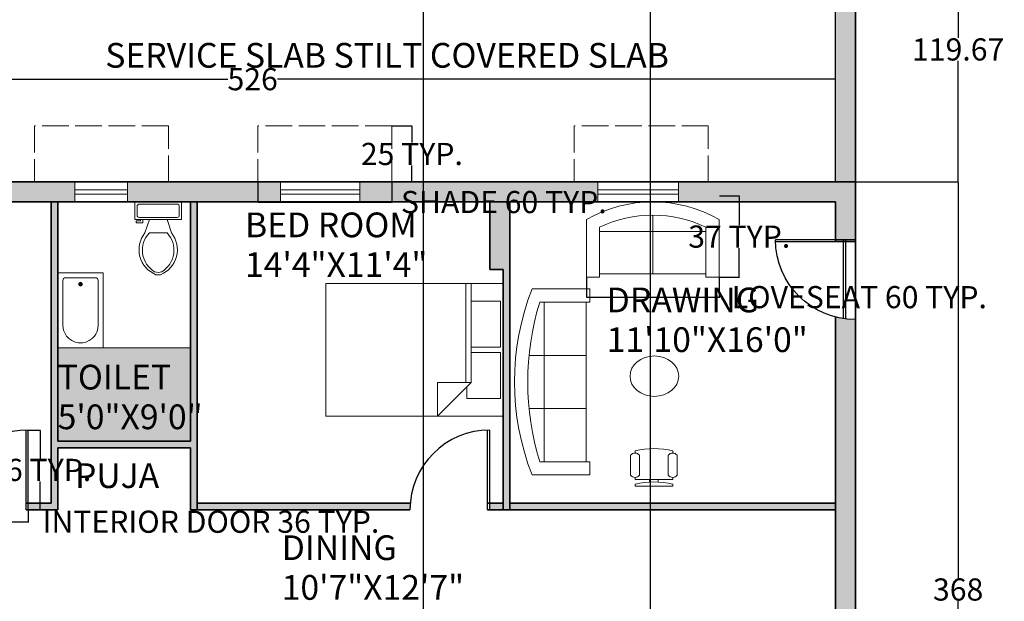
# Model space of a CAD drawing. Units: inches. Extents: x 215 to 969, y -612 to 418.
# Tile 3 of 8: x 502 to 947, y -356 to -93. Entities that reach past the tile are written whole.
import ezdxf

# ---------------------------------------------------------------- set-up
doc = ezdxf.new("R2010")
doc.units = ezdxf.units.IN
doc.header["$MEASUREMENT"] = 0
doc.linetypes.add('ACAD_ISO02W100', pattern=[15, 12, -3])
for name, color, linetype, lineweight in [('A-ANNO-DIMS', 2, 'Continuous', 18), ('A-ANNO-TEXT', 7, 'Continuous', 18), ('A-AREA-IDEN', 7, 'Continuous', 18), ('A-DOOR', 3, 'Continuous', 25), ('A-FLOR-FIXT', 9, 'Continuous', 18), ('A-FLOR-OVHD', 8, 'ACAD_ISO02W100', 13), ('A-FLOR-SLAB', 7, 'Continuous', 25), ('A-FURN', 8, 'Continuous', 18), ('A-GLAZ', 4, 'Continuous', 18), ('A-WALL', 7, 'Continuous', 35)]:
    doc.layers.add(name, color=color, linetype=linetype, lineweight=lineweight)
doc.layers.add('A-WALL-PATT', color=252, linetype='Continuous', lineweight=13, true_color=0x939598)
doc.styles.get("Standard").update_dxf_attribs({"font": 'arial.ttf'})
doc.dimstyles.get("Standard").update_dxf_attribs({"dimtxt": 10, "dimasz": 0.18, "dimexe": 0.18, "dimexo": 0.0625, "dimgap": 0.09, "dimtad": 0, "dimtih": 1, "dimtoh": 1, "dimdec": 0, "dimzin": 0, "dimdsep": 46, "dimlunit": 3, "dimtxsty": 'Standard', "dimcen": 0.09, "dimadec": 0, "dimazin": 0, "dimtfac": 1, "dimtdec": 0, "dimtofl": 0, "dimtmove": 0, "dimatfit": 3, "dimfxl": 1, "dimtolj": 1, "dimtzin": 0, "dimarcsym": 0})

# ---------------------------------------------------------------- blocks, each defined once
blk = doc.blocks.new('Toilet - top')
for p, q in [((9.5, -6), (9.5, -2)), ((-10, -8.5), (-8, -8.5)), ((-10, -9.5), (-10, -8.5)), ((-8, -8.5), (-8, -8)), ((-7, -8), (-7, -9.5)), ((-4, -8), (-6, -14)), ((4, -8), (6, -14)), ((-7, -9.5), (-10, -9.5)), ((4, -14), (-4, -14))]:
    blk.add_line(p, q)
blk.add_lwpolyline([(10.5, -8), (10.5, 0), (-10.5, 0), (-10.5, -8)], close=True)
for points in [[(-9.5, -2), (-9.5, -6)], [(8.5, -1), (-8.5, -1)], [(-8.5, -7), (8.5, -7)]]:
    blk.add_lwpolyline(points)
for centre, radius, start, end in [((-8.62, -1.88), 0.884, 81.8699, 188.1301), ((8.62, -1.88), 0.884, 351.8699, 98.1301), ((-8.62, -6.12), 0.884, 171.8699, 278.1301), ((8.62, -6.12), 0.884, 261.8699, 8.1301), ((3.52, -21.58), 12.17, 141.4691, 247.9714), ((4.2, -21.82), 11.33, 136.3677, 238.9468), ((-3.52, -21.58), 12.17, 292.0284, 38.5307), ((-4.2, -21.82), 11.33, 301.053, 43.6321), ((0, -27.88), 4, 245.7318, 294.2682), ((0, -29), 4, 254.8605, 285.1395)]:
    blk.add_arc(centre, radius, start, end)
blk = doc.blocks.new('Bath Tub - 26 x 60 in.')
for p, q in [((8, -18), (10, -18)), ((9, -17), (9, -19))]:
    blk.add_line(p, q)
blk.add_lwpolyline([(0, -36), (0, 0), (60, 0), (60, -36)], close=True)
for points in [[(4, -30), (4, -6)], [(6, -4), (42, -4)], [(42, -32), (6, -32)]]:
    blk.add_lwpolyline(points)
for radius in [1.5, 1]:
    blk.add_circle((9, -18), radius)
for centre, radius, start, end in [((5.75, -5.75), 1.77, 81.8699, 188.1301), ((42, -18), 14, 270, 90), ((5.75, -30.25), 1.77, 171.8699, 278.1301)]:
    blk.add_arc(centre, radius, start, end)
blk = doc.blocks.new('Bed - Queen')
for p, q in [((0, -80.00003), (0, 0)), ((0, 0), (59.99999, 0)), ((59.99999, 0), (59.99999, -80.00003)), ((7.99999, -1.2), (28.79998, -1.2)), ((7.99999, -14.4), (7.99999, -1.2)), ((28.79998, -1.2), (28.79998, -14.4)), ((31.19999, -1.2), (51.99999, -1.2)), ((31.19999, -14.4), (31.19999, -1.2)), ((51.99999, -1.2), (51.99999, -16.4)), ((0, -14.4), (44.8, -14.4)), ((44.8, -16.8), (0, -16.8)), ((59.99999, -29.6), (44.8, -14.4)), ((44.8, -14.4), (44.8, -29.6)), ((51.99999, -16.4), (46.79936, -16.4)), ((44.8, -29.6), (59.99999, -29.6)), ((59.99999, -80.00003), (0, -80.00003))]:
    blk.add_line(p, q)
blk = doc.blocks.new('Sofa - Roundback 7 ft.')
for p, q in [((-12.00002, -32.4421), (-12.00003, -6.5971)), ((11.99997, -32.4421), (11.99998, -6.5971)), ((-36.000027, -34), (-36.000027, -11.4696)), ((35.99998, -34), (35.99998, -11.4696)), ((-35.999844, -13.3819), (35.9998, -13.3819)), ((-36.000027, -32.4421), (35.99998, -32.4421))]:
    blk.add_line(p, q)
for points in [[(-36.000027, -34), (-42.000027, -34), (-42.000027, -8)], [(41.99998, -8), (41.99998, -34), (35.99998, -34)]]:
    blk.add_lwpolyline(points)
for centre, radius, start, end in [((0, -114.25), 114.25, 68.43141, 111.5686), ((-0.00001, -127.1968), 121.1968, 72.72033, 107.2797)]:
    blk.add_arc(centre, radius, start, end)
blk = doc.blocks.new('Sofa - Roundback Loveseat 5 ft.')
for p, q in [((0, -32.44198), (0, -5.99998)), ((-24, -33.99998), (-24, -11.46958)), ((24.00004, -33.99998), (24.00004, -11.46958)), ((-23.9998, -13.38178), (23.99986, -13.38178)), ((-24, -32.44198), (24.00004, -32.44198))]:
    blk.add_line(p, q)
for points in [[(-24, -33.99998), (-30, -33.99998), (-30, -7.99998)], [(30.00004, -7.99998), (30.00004, -33.99998), (24.00004, -33.99998)]]:
    blk.add_lwpolyline(points)
for centre, radius, start, end in [((0, -60.24998), 60.24998, 60.13715, 119.8628), ((0, -61.38438), 55.38444, 64.32083, 115.6792)]:
    blk.add_arc(centre, radius, start, end)
blk = doc.blocks.new('Chair - Desk')
for p, q in [((-8.5, 0), (-8.5, -1)), ((-8.5, 0), (8.5, 0)), ((8.5, 0), (8.5, -1)), ((-8.5, -3), (-8.5, -4)), ((-8.5, -3), (8.5, -3)), ((-2, -3), (-2, -1.9355)), ((2, -1.9576), (2, -3)), ((8.5, -3), (8.5, -4)), ((-10.5, -5), (-10.5, -14)), ((-6.5, -14), (-6.5, -5)), ((6.5, -5), (6.5, -14)), ((10.5, -14), (10.5, -5)), ((-8.5, -15), (-8.5, -16)), ((8.5, -15), (8.5, -16))]:
    blk.add_line(p, q)
for centre, radius, start, end in [((-8.5, -6.5), 2.5, 36.8699, 143.1301), ((0, 34.625), 36.625, 256.5803, 283.4197), ((8.5, -6.5), 2.5, 36.8699, 143.1301), ((-8.5, -12.5), 2.5, 216.8699, 323.1301), ((0, 19.625), 36.625, 256.5803, 283.4197), ((8.5, -12.5), 2.5, 216.8699, 323.1301)]:
    blk.add_arc(centre, radius, start, end)
blk = doc.blocks.new('WINDOW-SHADE-60')
for p, q in [((60.48, 25.28), (0, 25.28)), ((0, 25.28), (0, 0)), ((60.48, 0), (60.48, 25.28))]:
    blk.add_line(p, q)
blk = doc.blocks.new('DOOR-SINGLE-36')
for p, q in [((35, 0), (35, 36)), ((36, 0), (36, 36)), ((35, 0), (36, 0))]:
    blk.add_line(p, q)
blk.add_arc((36, 0), 36, 90, 180)
blk = doc.blocks.new('DOOR-ENTRY-36')
for p, q in [((36, 1), (0, 1)), ((36, 0), (0, 0))]:
    blk.add_line(p, q)
blk.add_arc((36, 0), 36, 90, 180)
blk = doc.blocks.new('WIN-FRAME-24A')
for p, q in [((0, 0), (0, 9)), ((23.77, 0), (23.77, 9)), ((23.77, 5.5), (0, 5.5)), ((0, 4.5), (0, 0)), ((23.77, 3.5), (0, 3.5))]:
    blk.add_line(p, q)
blk = doc.blocks.new('WIN-FRAME-36A')
for p, q in [((0, 35.94), (9, 35.94)), ((3.5, 35.94), (3.5, 0)), ((5.5, 35.94), (5.5, 0)), ((9, 0), (0, 0)), ((4.5, 0), (9, 0))]:
    blk.add_line(p, q)
blk = doc.blocks.new('WIN-FRAME-36B')
for p, q in [((9, 36.42), (0, 36.42)), ((3.5, 36.42), (3.5, 0)), ((5.5, 36.42), (5.5, 0)), ((4.5, 0), (0, 0)), ((0, 0), (9, 0))]:
    blk.add_line(p, q)
blk = doc.blocks.new('*D37')
at = {"layer": 'A-ANNO-DIMS', "color": 0, "lineweight": -2, "transparency": 16777216}
for p, q in [((609.64, -166.51), (609.64, -175.7)), ((670.12, -166.51), (670.12, -175.7)), ((609.82, -175.52), (669.94, -175.52)), ((670.12, -175.52), (670.3, -175.52))]:
    blk.add_line(p, q, dxfattribs=at)
at = {"layer": 'A-ANNO-DIMS', "color": 0, "transparency": 16777216}
for points in [[(609.82, -175.49), (609.82, -175.55), (609.64, -175.52)], [(669.94, -175.49), (669.94, -175.55), (670.12, -175.52)]]:
    blk.add_solid(points, dxfattribs=at)
at = {"layer": 'Defpoints', "color": 0, "transparency": 16777216}
for p in [(609.64, -166.45), (670.12, -166.45), (670.12, -175.52)]:
    blk.add_point(p, dxfattribs=at)
at = {"layer": 'A-ANNO-DIMS', "color": 0, "transparency": 16777216, "insert": (720.71, -175.52), "char_height": 10, "attachment_point": 5}
blk.add_mtext('\\A1;SHADE 60 TYP.', dxfattribs=at)
blk = doc.blocks.new('*D38')
at = {"layer": 'A-ANNO-DIMS', "color": 0, "lineweight": -2, "transparency": 16777216}
for p, q in [((670.19, -141.18), (679.38, -141.18)), ((679.2, -141.36), (679.2, -148.62)), ((679.2, -166.27), (679.2, -159.01)), ((670.19, -166.45), (679.38, -166.45))]:
    blk.add_line(p, q, dxfattribs=at)
at = {"layer": 'A-ANNO-DIMS', "color": 0, "transparency": 16777216}
for points in [[(679.17, -141.36), (679.23, -141.36), (679.2, -141.18)], [(679.17, -166.27), (679.23, -166.27), (679.2, -166.45)]]:
    blk.add_solid(points, dxfattribs=at)
at = {"layer": 'Defpoints', "color": 0, "transparency": 16777216}
for p in [(670.12, -141.18), (679.2, -141.18), (670.12, -166.45)]:
    blk.add_point(p, dxfattribs=at)
at = {"layer": 'A-ANNO-DIMS', "color": 0, "transparency": 16777216, "insert": (679.2, -153.81), "char_height": 10, "attachment_point": 5}
blk.add_mtext('\\A1;25 TYP.', dxfattribs=at)
blk = doc.blocks.new('*D39')
at = {"layer": 'A-ANNO-DIMS', "color": 0, "lineweight": -2, "transparency": 16777216}
for p, q in [((470.07, -314.51), (470.07, -320.03)), ((506.07, -314.51), (506.07, -320.03)), ((470.25, -319.85), (505.89, -319.85)), ((506.07, -319.85), (506.25, -319.85))]:
    blk.add_line(p, q, dxfattribs=at)
at = {"layer": 'A-ANNO-DIMS', "color": 0, "transparency": 16777216}
for points in [[(470.25, -319.82), (470.25, -319.88), (470.07, -319.85)], [(505.89, -319.82), (505.89, -319.88), (506.07, -319.85)]]:
    blk.add_solid(points, dxfattribs=at)
at = {"layer": 'Defpoints', "color": 0, "transparency": 16777216}
for p in [(470.07, -314.45), (506.07, -314.45), (506.07, -319.85)]:
    blk.add_point(p, dxfattribs=at)
at = {"layer": 'A-ANNO-DIMS', "color": 0, "transparency": 16777216, "insert": (588.53, -319.85), "char_height": 10, "attachment_point": 5}
blk.add_mtext('\\A1;INTERIOR DOOR 36 TYP.', dxfattribs=at)
blk = doc.blocks.new('*D40')
at = {"layer": 'A-ANNO-DIMS', "color": 0, "lineweight": -2, "transparency": 16777216}
for p, q in [((506.13, -278.45), (511.65, -278.45)), ((511.47, -278.63), (511.47, -291.25)), ((511.47, -314.27), (511.47, -301.65)), ((506.13, -314.45), (511.65, -314.45))]:
    blk.add_line(p, q, dxfattribs=at)
at = {"layer": 'A-ANNO-DIMS', "color": 0, "transparency": 16777216}
for points in [[(511.44, -278.63), (511.5, -278.63), (511.47, -278.45)], [(511.44, -314.27), (511.5, -314.27), (511.47, -314.45)]]:
    blk.add_solid(points, dxfattribs=at)
at = {"layer": 'Defpoints', "color": 0, "transparency": 16777216}
for p in [(506.07, -278.45), (511.47, -278.45), (506.07, -314.45)]:
    blk.add_point(p, dxfattribs=at)
at = {"layer": 'A-ANNO-DIMS', "color": 0, "transparency": 16777216, "insert": (511.47, -296.45), "char_height": 10, "attachment_point": 5}
blk.add_mtext('\\A1;36 TYP.', dxfattribs=at)
blk = doc.blocks.new('*D43')
at = {"layer": 'A-ANNO-DIMS', "color": 0, "lineweight": -2, "transparency": 16777216}
for p, q in [((757.95, -209.51), (757.95, -218.63)), ((817.95, -209.51), (817.95, -218.63)), ((758.13, -218.45), (817.77, -218.45)), ((817.95, -218.45), (818.13, -218.45))]:
    blk.add_line(p, q, dxfattribs=at)
at = {"layer": 'A-ANNO-DIMS', "color": 0, "transparency": 16777216}
for points in [[(758.13, -218.42), (758.13, -218.48), (757.95, -218.45)], [(817.77, -218.42), (817.77, -218.48), (817.95, -218.45)]]:
    blk.add_solid(points, dxfattribs=at)
at = {"layer": 'Defpoints', "color": 0, "transparency": 16777216}
for p in [(757.95, -209.45), (817.95, -209.45), (817.95, -218.45)]:
    blk.add_point(p, dxfattribs=at)
at = {"layer": 'A-ANNO-DIMS', "color": 0, "transparency": 16777216, "insert": (881.15, -218.45), "char_height": 10, "attachment_point": 5}
blk.add_mtext('\\A1;LOVESEAT 60 TYP.', dxfattribs=at)
blk = doc.blocks.new('*D44')
at = {"layer": 'A-ANNO-DIMS', "color": 0, "lineweight": -2, "transparency": 16777216}
for p, q in [((818.01, -172.79), (827.13, -172.79)), ((826.95, -172.97), (826.95, -185.92)), ((826.95, -209.27), (826.95, -196.32)), ((818.01, -209.45), (827.13, -209.45))]:
    blk.add_line(p, q, dxfattribs=at)
at = {"layer": 'A-ANNO-DIMS', "color": 0, "transparency": 16777216}
for points in [[(826.92, -172.97), (826.98, -172.97), (826.95, -172.79)], [(826.92, -209.27), (826.98, -209.27), (826.95, -209.45)]]:
    blk.add_solid(points, dxfattribs=at)
at = {"layer": 'Defpoints', "color": 0, "transparency": 16777216}
for p in [(817.95, -172.79), (826.95, -172.79), (817.95, -209.45)]:
    blk.add_point(p, dxfattribs=at)
at = {"layer": 'A-ANNO-DIMS', "color": 0, "transparency": 16777216, "insert": (826.95, -191.12), "char_height": 10, "attachment_point": 5}
blk.add_mtext('\\A1;37 TYP.', dxfattribs=at)
blk = doc.blocks.new('*D69')
at = {"layer": 'A-ANNO-DIMS', "color": 0, "lineweight": -2, "transparency": 16777216}
for p, q in [((344.35, -166.39), (344.35, -119.87)), ((870.35, -166.39), (870.35, -119.87)), ((344.53, -120.05), (596.22, -120.05)), ((870.17, -120.05), (618.49, -120.05))]:
    blk.add_line(p, q, dxfattribs=at)
at = {"layer": 'A-ANNO-DIMS', "color": 0, "transparency": 16777216}
for points in [[(344.53, -120.02), (344.53, -120.08), (344.35, -120.05)], [(870.17, -120.02), (870.17, -120.08), (870.35, -120.05)]]:
    blk.add_solid(points, dxfattribs=at)
at = {"layer": 'Defpoints', "color": 0, "transparency": 16777216}
for p in [(870.35, -120.05), (344.35, -166.45), (870.35, -166.45)]:
    blk.add_point(p, dxfattribs=at)
at = {"layer": 'A-ANNO-DIMS', "color": 0, "transparency": 16777216, "insert": (607.35, -120.05), "char_height": 10, "attachment_point": 5}
blk.add_mtext('\\A1;526', dxfattribs=at)
blk = doc.blocks.new('*D71')
at = {"layer": 'A-ANNO-DIMS', "color": 0, "lineweight": -2, "transparency": 16777216}
for p, q in [((879.42, -46.79), (925.93, -46.79)), ((925.75, -46.97), (925.75, -101.42)), ((925.75, -166.27), (925.75, -111.82)), ((879.42, -166.45), (925.93, -166.45))]:
    blk.add_line(p, q, dxfattribs=at)
at = {"layer": 'A-ANNO-DIMS', "color": 0, "transparency": 16777216}
for points in [[(925.72, -46.97), (925.78, -46.97), (925.75, -46.79)], [(925.72, -166.27), (925.78, -166.27), (925.75, -166.45)]]:
    blk.add_solid(points, dxfattribs=at)
at = {"layer": 'Defpoints', "color": 0, "transparency": 16777216}
for p in [(879.35, -46.79), (879.35, -166.45), (925.75, -166.45)]:
    blk.add_point(p, dxfattribs=at)
at = {"layer": 'A-ANNO-DIMS', "color": 0, "transparency": 16777216, "insert": (925.75, -106.62), "char_height": 10, "attachment_point": 5}
blk.add_mtext('\\A1;119.67', dxfattribs=at)
blk = doc.blocks.new('*D72')
at = {"layer": 'A-ANNO-DIMS', "color": 0, "lineweight": -2, "transparency": 16777216}
for p, q in [((879.42, -166.45), (925.93, -166.45)), ((925.75, -166.63), (925.75, -345.25)), ((925.75, -534.27), (925.75, -355.65)), ((879.42, -534.45), (925.93, -534.45))]:
    blk.add_line(p, q, dxfattribs=at)
at = {"layer": 'A-ANNO-DIMS', "color": 0, "transparency": 16777216}
for points in [[(925.72, -166.63), (925.78, -166.63), (925.75, -166.45)], [(925.72, -534.27), (925.78, -534.27), (925.75, -534.45)]]:
    blk.add_solid(points, dxfattribs=at)
at = {"layer": 'Defpoints', "color": 0, "transparency": 16777216}
for p in [(879.35, -166.45), (879.35, -534.45), (925.75, -534.45)]:
    blk.add_point(p, dxfattribs=at)
at = {"layer": 'A-ANNO-DIMS', "color": 0, "transparency": 16777216, "insert": (925.75, -350.45), "char_height": 10, "attachment_point": 5}
blk.add_mtext('\\A1;368', dxfattribs=at)
blk = doc.blocks.new('*D75')
at = {"layer": 'A-ANNO-DIMS', "color": 0, "lineweight": -2, "transparency": 16777216}
for p, q in [((290.35, 103.15), (290.35, -605.89)), ((879.35, -534.51), (879.35, -605.89)), ((290.53, -605.71), (573.71, -605.71)), ((879.17, -605.71), (596, -605.71))]:
    blk.add_line(p, q, dxfattribs=at)
at = {"layer": 'A-ANNO-DIMS', "color": 0, "transparency": 16777216}
for points in [[(290.53, -605.68), (290.53, -605.74), (290.35, -605.71)], [(879.17, -605.68), (879.17, -605.74), (879.35, -605.71)]]:
    blk.add_solid(points, dxfattribs=at)
at = {"layer": 'Defpoints', "color": 0, "transparency": 16777216}
for p in [(290.35, 103.21), (879.35, -534.45), (879.35, -605.71)]:
    blk.add_point(p, dxfattribs=at)
at = {"layer": 'A-ANNO-DIMS', "color": 0, "transparency": 16777216, "insert": (584.85, -605.71), "char_height": 10, "attachment_point": 5}
blk.add_mtext('\\A1;589', dxfattribs=at)
blk = doc.blocks.new('*D76')
at = {"layer": 'A-ANNO-DIMS', "color": 0, "lineweight": -2, "transparency": 16777216}
for p, q in [((569.29, 365.5), (243.77, 365.5)), ((243.95, 365.32), (243.95, -91.71)), ((243.95, -559.13), (243.95, -102.1)), ((454.66, -559.31), (243.77, -559.31))]:
    blk.add_line(p, q, dxfattribs=at)
at = {"layer": 'A-ANNO-DIMS', "color": 0, "transparency": 16777216}
for points in [[(243.92, 365.32), (243.98, 365.32), (243.95, 365.5)], [(243.92, -559.13), (243.98, -559.13), (243.95, -559.31)]]:
    blk.add_solid(points, dxfattribs=at)
at = {"layer": 'Defpoints', "color": 0, "transparency": 16777216}
for p in [(569.35, 365.5), (243.95, -559.31), (454.72, -559.31)]:
    blk.add_point(p, dxfattribs=at)
at = {"layer": 'A-ANNO-DIMS', "color": 0, "transparency": 16777216, "insert": (243.95, -96.91), "char_height": 10, "attachment_point": 5}
blk.add_mtext('\\A1;924.8', dxfattribs=at)
blk = doc.blocks.new('*D79')
at = {"layer": 'A-ANNO-DIMS', "color": 0, "lineweight": -2, "transparency": 16777216}
for p, q in [((684.35, -82.85), (684.35, -605.89)), ((786.74, -82.85), (786.74, -605.89)), ((684.53, -605.71), (715.16, -605.71)), ((786.56, -605.71), (755.93, -605.71))]:
    blk.add_line(p, q, dxfattribs=at)
at = {"layer": 'A-ANNO-DIMS', "color": 0, "transparency": 16777216}
for points in [[(684.53, -605.68), (684.53, -605.74), (684.35, -605.71)], [(786.56, -605.68), (786.56, -605.74), (786.74, -605.71)]]:
    blk.add_solid(points, dxfattribs=at)
at = {"layer": 'Defpoints', "color": 0, "transparency": 16777216}
for p in [(684.35, -82.79), (786.74, -82.79), (786.74, -605.71)]:
    blk.add_point(p, dxfattribs=at)
at = {"layer": 'A-ANNO-DIMS', "color": 0, "transparency": 16777216, "insert": (735.55, -605.71), "char_height": 10, "attachment_point": 5}
blk.add_mtext('\\A1;102.38', dxfattribs=at)
blk = doc.blocks.new('*D81')
at = {"layer": 'A-ANNO-DIMS', "color": 0, "lineweight": -2, "transparency": 16777216}
for p, q in [((786.74, -46.85), (786.74, -605.89)), ((879.35, -46.85), (879.35, -605.89)), ((786.92, -605.71), (816.13, -605.71)), ((879.17, -605.71), (849.96, -605.71))]:
    blk.add_line(p, q, dxfattribs=at)
at = {"layer": 'A-ANNO-DIMS', "color": 0, "transparency": 16777216}
for points in [[(786.92, -605.68), (786.92, -605.74), (786.74, -605.71)], [(879.17, -605.68), (879.17, -605.74), (879.35, -605.71)]]:
    blk.add_solid(points, dxfattribs=at)
at = {"layer": 'Defpoints', "color": 0, "transparency": 16777216}
for p in [(786.74, -46.79), (879.35, -46.79), (879.35, -605.71)]:
    blk.add_point(p, dxfattribs=at)
at = {"layer": 'A-ANNO-DIMS', "color": 0, "transparency": 16777216, "insert": (833.05, -605.71), "char_height": 10, "attachment_point": 5}
blk.add_mtext('\\A1;92.62', dxfattribs=at)

msp = doc.modelspace()

# ---------------------------------------------------------------- hatches: boundary and pattern name
at = {"layer": 'A-WALL-PATT'}
h = msp.add_hatch(color=256, dxfattribs=at)
h.dxf.hatch_style = 1
h.paths.add_polyline_path([(764.0736, 322.2135), (569.3535, 322.2135), (565.0643, 322.2135), (565.0643, 313.2135), (569.3535, 313.2135), (569.3535, 205.2135), (509.3535, 205.2135), (509.3535, 247.2592), (506.3535, 247.2592), (506.3535, 172.2135), (491.3535, 172.2135), (491.3535, 169.2135), (509.3535, 169.2135), (509.3535, 202.2135), (569.3535, 202.2135), (569.3535, 169.2135), (578.3535, 169.2135), (578.3535, 205.2135), (578.3535, 237.2135), (615.7789, 237.2135), (615.7789, 246.2135), (578.3535, 246.2135), (578.3535, 313.2135), (710.3535, 313.2135), (710.3535, 246.2135), (710.3535, 211.3874), (719.3535, 211.3874), (719.3535, 295.2135), (719.3535, 313.2135), (764.0736, 313.2135)])
h.paths.add_polyline_path([(879.3535, 322.2135), (811.6486, 322.2135), (811.6486, 313.2135), (870.3535, 313.2135), (870.3535, 215.3905, -0.06325422), (879.3535, 216.5337), (879.3535, 313.2135)])
h.paths.add_polyline_path([(879.3535, 157.2135), (879.3535, 180.5337), (870.3535, 180.5337), (870.3535, 157.2135), (719.3535, 157.2135), (710.3535, 157.2135), (710.3535, 148.2135), (719.3535, 148.2135), (870.3535, 148.2135), (870.3535, 16.2135), (838.4933, 16.2135), (838.4933, 13.2135), (870.3535, 13.2135), (870.3535, -37.7865), (844.0345, -37.7865), (844.0345, -46.7865), (870.3535, -46.7865), (879.3535, -46.7865), (879.3535, -37.7865), (879.3535, 137.613)])
h.paths.add_polyline_path([(710.3535, 246.2135), (663.4146, 246.2135), (663.4146, 237.2135), (710.3535, 237.2135)], flags=17)
h.paths.add_polyline_path([(541.2942, 322.2135), (509.3535, 322.2135), (468.3222, 322.2135), (468.3222, 313.2135), (500.3535, 313.2135), (509.3535, 313.2135), (541.2942, 313.2135)])
h.paths.add_polyline_path([(509.3535, 313.2135), (503.3535, 313.2135), (503.3535, 277.5241, -0.04952579), (509.3535, 277.4203)], flags=17)
h.paths.add_polyline_path([(420.2828, 322.2135), (335.3535, 322.2135), (335.3535, 235.2487), (344.3535, 235.2487), (344.3535, 284.1885), (344.3535, 313.2135), (420.2828, 313.2135)])
h.paths.add_polyline_path([(335.3535, 181.2135), (290.3535, 181.2135), (290.3535, 103.2135), (335.3535, 103.2135), (335.3535, 112.2135), (299.3535, 112.2135), (299.3535, 129.1615), (299.3535, 172.2135), (335.3535, 172.2135)])
h.paths.add_polyline_path([(344.3535, 199.3097), (335.3535, 199.3097), (335.3535, 172.2135), (335.3535, 157.3369), (344.3535, 157.3369), (344.3535, 169.2135), (452.3535, 169.2135), (452.5037, 169.2135), (452.5037, 150.1199), (452.3535, 109.2135), (455.3535, 109.2135), (455.3535, 169.2135, -0.02086055), (455.4787, 172.2135), (344.3535, 172.2135)])
h.paths.add_polyline_path([(344.3535, 133.3441), (335.3535, 133.3441), (335.3535, 77.89), (344.3535, 77.89), (344.3535, 103.2135), (401.3556, 103.2135), (401.3556, 109.2135), (344.3535, 109.2135)])
h.paths.add_polyline_path([(462.6362, 109.2135), (443.0437, 109.2135), (425.2018, 109.2135), (425.2018, 106.2135), (452.3535, 106.2135), (462.7615, 106.2135, -0.02086055)])
h.paths.add_polyline_path([(540.3535, 106.2135), (684.3535, 106.2135), (684.3535, 35.7135), (687.3535, 35.7135), (687.3535, 56.1856), (693.3535, 56.1856), (693.3535, 109.2135), (540.3535, 109.2135), (531.3535, 109.2135), (498.6362, 109.2135), (498.6362, 106.2135), (531.3535, 106.2135), (531.3535, -37.7865), (507.9524, -37.7865), (507.9524, -46.7865), (610.6038, -46.7865), (610.6038, -37.7865), (540.3535, -37.7865)])
h.paths.add_polyline_path([(578.3535, 358.6622), (555.879, 358.6622), (555.879, 349.6622), (569.3535, 349.6622), (569.3535, 322.2135), (578.3535, 322.2135)])
h.paths.add_polyline_path([(525.962, 358.6622), (503.3535, 358.6622), (503.3535, 322.2135), (509.3535, 322.2135), (509.3535, 349.6622), (525.962, 349.6622)])
h.paths.add_polyline_path([(344.3535, 30.022), (335.3535, 30.022), (335.3535, -37.7865), (335.3535, -46.7865), (484.3302, -46.7865), (484.3302, -37.7865), (344.3535, -37.7865)])
h.paths.add_polyline_path([(719.1188, -37.7865), (698.4193, -37.7865), (693.3535, -37.7865), (693.3535, 7.424, -0.07717369), (684.3535, 6.0404), (684.3535, -37.7865), (658.8269, -37.7865), (658.8269, -46.7865), (684.3535, -46.7865), (684.3535, -82.7865), (693.3535, -82.7865), (704.1236, -82.7865), (704.1236, -78.0462), (693.3535, -78.0462), (693.3535, -46.7865), (719.1188, -46.7865)])
h.paths.add_polyline_path([(684.3535, -14.2202), (669.6716, -14.2202), (669.6716, -16.6044, -0.23606798), (667.6716, -17.6044), (667.6716, -18.6044, -0.11764706), (650.6716, -18.6044), (650.6716, -17.6044, -0.23606798), (648.6716, -16.6044), (648.6716, -14.2202), (603.0565, -14.2202), (603.0565, -37.7865), (684.3535, -37.7865)], flags=17)
h.paths.add_polyline_path([(665.6716, -14.2202), (652.6716, -14.2202), (652.6716, -16.6044, -0.23606798), (650.6716, -17.6044), (650.6716, -18.6044, 0.11764706), (667.6716, -18.6044), (667.6716, -17.6044, -0.23606798), (665.6716, -16.6044)], flags=16)
h.paths.add_polyline_path([(786.7385, -37.7865), (755.3535, -37.7865), (755.3535, 13.2135), (769.0808, 13.2135), (769.0808, 16.2135), (755.3535, 16.2135), (755.3535, 73.2135), (753.3535, 73.2135), (693.3535, 73.2135), (693.3535, 70.2135), (753.3535, 70.2135), (753.3535, -37.7865), (743.3062, -37.7865), (743.3062, -46.7865), (781.7385, -46.7865), (781.7385, -82.7865), (786.7385, -82.7865), (786.7385, -82.3744), (786.7385, -46.7865)])
h.paths.add_polyline_path([(844.0345, -37.7865), (786.7385, -37.7865), (786.7385, -46.7865), (844.0345, -46.7865)], flags=17)
h.paths.add_polyline_path([(781.7385, -78.0462), (704.1236, -78.0462), (704.1236, -82.7865), (781.7385, -82.7865)], flags=17)
h.paths.add_polyline_path([(344.3535, -46.7865), (335.3535, -46.7865), (335.3535, -166.4525), (344.3535, -166.4525)])
h.paths.add_polyline_path([(382.6632, 103.2135), (344.3535, 103.2135), (344.3535, 77.89), (344.3535, 32.7135), (363.5083, 32.7135), (382.6632, 32.7135)])
h.paths.add_polyline_path([(879.3535, -46.7865), (870.3535, -46.7865), (870.3535, -166.4525), (879.3535, -166.4525)])
h.paths.add_polyline_path([(879.3535, -166.4525), (799.4745, -166.4525), (799.4745, -175.4525), (855.3535, -175.4525), (870.3535, -175.4525), (870.3535, -192.5449), (879.3535, -192.5449), (879.3535, -175.4525)])
h.paths.add_polyline_path([(763.1775, -166.4525), (655.7214, -166.4525), (655.7214, -175.4525), (763.1775, -175.4525)])
h.paths.add_polyline_path([(619.8538, -166.4525), (550.8369, -166.4525), (550.8369, -175.4525), (619.8538, -175.4525)])
h.paths.add_polyline_path([(527.1282, -166.4525), (427.0819, -166.4525), (427.0819, -175.4525), (527.1282, -175.4525)])
h.paths.add_polyline_path([(391.4021, -166.4525), (335.3535, -166.4525), (335.3535, -175.4525), (335.3535, -236.0109), (344.3535, -236.0109), (344.3535, -187.5037), (344.3535, -175.4525), (391.4021, -175.4525)])
h.paths.add_polyline_path([(344.3535, -271.9249), (335.3535, -271.9249), (335.3535, -331.0209), (344.3535, -331.0209), (344.3535, -314.4525), (412.4218, -314.4525, -0.02503209), (412.3073, -311.4525), (344.3535, -311.4525)])
h.paths.add_polyline_path([(470.1954, -311.4525), (442.3073, -311.4525), (442.3073, -314.4525), (470.0702, -314.4525, -0.02086055)])
h.paths.add_polyline_path([(455.3535, -314.4525), (452.3535, -314.4525), (452.3535, -374.4525), (455.3535, -374.4525)])
h.paths.add_polyline_path([(579.3535, -241.4072), (519.3535, -241.4072), (519.3535, -283.4525), (579.3535, -283.4525)])
h.paths.add_polyline_path([(516.5043, -281.1089), (584.3098, -281.1089), (584.3098, -264.0138), (516.5043, -264.0138)], flags=9)
h.paths.add_polyline_path([(516.4662, -263.2183), (581.1504, -263.2183), (581.1504, -245.8948), (516.4662, -245.8948)], flags=9)
h = msp.add_hatch(color=256, dxfattribs=at)
h.dxf.hatch_style = 1
h.paths.add_polyline_path([(723.3535, -175.4525), (714.3535, -175.4525), (714.3535, -205.9065), (720.3535, -205.9065), (720.3535, -314.4525), (723.3535, -314.4525)])
h.paths.add_polyline_path([(720.3535, -311.4525), (714.3535, -311.4525), (714.3535, -314.4525), (720.3535, -314.4525)], flags=17)
h.paths.add_polyline_path([(879.3535, -228.5449, -0.06325422), (870.3535, -227.4017), (870.3535, -314.4525), (870.3535, -410.4525), (870.3535, -464.8456), (870.3535, -525.4525), (730.3535, -525.4525), (730.3535, -473.8456), (753.1403, -473.8456), (753.1403, -464.8456), (686.9324, -464.8456), (686.9324, -473.8456), (721.3535, -473.8456), (721.3535, -525.4525), (594.3535, -525.4525), (594.3535, -473.8456), (622.1543, -473.8456), (622.1543, -464.8456), (594.3535, -464.8456), (594.3535, -414.4525), (525.3535, -414.4525), (525.3535, -417.4525), (585.3535, -417.4525), (585.3535, -525.4525), (571.9682, -525.4525), (571.9682, -534.4525), (879.3535, -534.4525), (879.3535, -410.4525), (879.3535, -314.4525)])
h.paths.add_polyline_path([(730.3535, -368.8456), (870.3535, -368.8456), (870.3535, -365.8456), (721.3535, -365.8456), (721.3535, -368.8456), (721.3535, -409.1143), (730.3535, -409.1143)], flags=17)
h.paths.add_polyline_path([(870.3535, -410.4525), (870.3535, -368.8456), (763.5487, -368.8456), (763.5487, -393.1792), (831.3894, -393.1792), (831.3894, -438.7284), (789.7386, -438.7284), (789.7386, -464.8456), (870.3535, -464.8456)], flags=17)
h.paths.add_polyline_path([(839.0857, -434.8848), (839.0857, -399.5193), (865.1757, -399.5193), (865.1757, -434.8848)], flags=16)
h.paths.add_polyline_path([(839.8092, -427.6923, -0.48074962), (841.3551, -426.456, -0.48074962), (842.901, -427.6923, -0.48074962), (841.3551, -428.9285, -0.48074962)], flags=0)
h.paths.add_polyline_path([(848.5001, -427.1588, -0.44021274), (854.7228, -421.4606, -0.49540019), (861.9637, -426.9752, -0.44021274), (855.741, -432.6734, -0.49540019)], flags=0)
h.paths.add_polyline_path([(848.5001, -410.0762, -0.44021274), (854.7228, -404.378, -0.49540019), (861.9637, -409.8925, -0.44021274), (855.741, -415.5907, -0.49540019)], flags=0)
h.paths.add_polyline_path([(839.8092, -410.149, -0.48074962), (841.3551, -408.9127, -0.48074962), (842.901, -410.149, -0.48074962), (841.3551, -411.3852, -0.48074962)], flags=0)
h.paths.add_polyline_path([(870.3535, -464.8456), (789.7386, -464.8456), (789.1403, -464.8456, -0.06325422), (787.9971, -473.8456), (870.3535, -473.8456)], flags=17)
h.paths.add_polyline_path([(727.9401, -444.9303), (724.3796, -444.9303), (724.3796, -464.8456), (727.9401, -464.8456)], flags=17)
h.paths.add_polyline_path([(548.597, -525.4525), (531.2503, -525.4525), (525.3535, -525.4525), (525.3535, -490.3641, -0.07632083), (516.3535, -491.7459), (516.3535, -525.4525), (488.9462, -525.4525), (488.9462, -534.4525), (548.597, -534.4525)])
h.paths.add_polyline_path([(525.3535, -374.4525), (506.0702, -374.4525), (506.0702, -377.4525), (516.3535, -377.4525), (516.3535, -461.7459), (519.3535, -461.7459), (519.3535, -417.4525), (525.3535, -417.4525), (525.3535, -414.4525)])
h.paths.add_polyline_path([(470.1724, -377.4525), (449.6899, -377.4525), (344.3535, -377.4525), (344.3535, -400.7118), (335.3535, -400.7118), (335.3535, -355.0472), (344.3535, -355.0472), (344.3535, -374.4525), (373.6368, -374.4525), (373.6368, -366.4525), (380.1368, -366.4525), (378.1369, -360.4526, -0.50132349), (383.0921, -341.5914, -0.13289091), (385.1815, -341.5914, -0.50131678), (390.1369, -360.4524), (388.1368, -366.4525), (391.1368, -366.4525), (391.1368, -364.9525), (394.1368, -364.9525), (394.1368, -365.9525), (392.1368, -365.9525), (392.1368, -366.4525), (394.6368, -366.4525), (394.6368, -374.4525), (418.4066, -374.4525), (418.4066, -354.0926), (452.3535, -354.0926), (452.3535, -374.4525), (470.0713, -374.4525, 0.02085422)])
h.paths.add_polyline_path([(442.1598, -372.1903), (421.7999, -372.1903, -0.50000012), (420.6688, -371.0592), (420.6688, -357.4859, -0.50000012), (421.7999, -356.3548), (442.1598, -356.3548, -1)], flags=16)
h.paths.add_polyline_path([(422.6483, -364.2725, -1), (424.3449, -364.2725, -1)], flags=0)
h.paths.add_polyline_path([(422.931, -364.2725, -1), (424.0621, -364.2725, -1)], flags=0)
h.paths.add_polyline_path([(392.6368, -373.4525), (375.6368, -373.4525, -0.50000012), (374.6368, -372.4525), (374.6368, -368.4525, -0.50000012), (375.6368, -367.4525), (392.6368, -367.4525, -0.50000012), (393.6368, -368.4525), (393.6368, -372.4525, -0.50000012)], flags=16)
h.paths.add_polyline_path([(388.1368, -360.4525), (380.1368, -360.4525, -0.4800795), (382.4928, -342.9295, -0.21500378), (385.7809, -342.9295, -0.48007965)], flags=16)
h.paths.add_polyline_path([(344.3535, -437.1356), (335.3535, -437.1356), (335.3535, -525.4525), (335.3535, -534.4525), (465.575, -534.4525), (465.575, -525.4525), (344.3535, -525.4525)])
h.paths.add_polyline_path([(342.2824, -347.0067), (391.5718, -347.0067), (391.5718, -334.5799), (342.2824, -334.5799)], flags=9)
h = msp.add_hatch(color=256, dxfattribs=at)
h.dxf.hatch_style = 1
h.paths.add_polyline_path([(678.4787, -311.4525), (582.3535, -311.4525), (582.3535, -314.4525), (678.3535, -314.4525, -0.02086055)])
h.paths.add_polyline_path([(582.3535, -283.4525), (582.3535, -175.4525), (579.3535, -175.4525), (579.3535, -283.4525), (519.3535, -283.4525), (519.3535, -175.4525), (516.3535, -175.4525), (516.3535, -311.4525), (506.0702, -311.4525), (506.0702, -314.4525), (519.3535, -314.4525), (519.3535, -286.4525), (579.3535, -286.4525), (579.3535, -314.4525), (582.3535, -314.4525), (582.3535, -311.4525)])
h.paths.add_polyline_path([(870.3535, -311.4525), (723.3535, -311.4525), (723.3535, -314.4525), (870.3535, -314.4525)])
h.paths.add_polyline_path([(516.5043, -281.1089), (584.3098, -281.1089), (584.3098, -264.0138), (516.5043, -264.0138)], flags=9)

# ---------------------------------------------------------------- linework, layer by layer
at = {"layer": 'A-DOOR'}
for p, q in [((870.3535, -192.5449), (879.3535, -192.5449)), ((873.8535, -192.5449), (873.8535, -228.1222)), ((874.8535, -192.5449), (874.8535, -228.2625)), ((879.3535, -192.5449), (879.3535, -228.5449)), ((506.0702, -314.4525), (506.0702, -311.4525)), ((714.3535, -314.4525), (714.3535, -311.4525))]:
    msp.add_line(p, q, dxfattribs=at)
at = {"layer": 'A-FLOR-FIXT'}
msp.add_line((519.493, -241.4072), (579.3535, -241.4072), dxfattribs=at)
at = {"layer": 'A-FLOR-SLAB'}
for p, q in [((870.3535, -166.4525), (870.3535, -46.7865)), ((879.3535, -175.4525), (879.3535, -46.7865))]:
    msp.add_line(p, q, dxfattribs=at)
at = {"layer": 'A-FURN'}
msp.add_ellipse((788.639, -254.1412), major_axis=(-10.9882, 0), ratio=0.83003055, dxfattribs=at)
at = {"layer": 'A-WALL'}
for p, q in [((335.3535, -166.4525), (879.3535, -166.4525)), ((344.3535, -175.4525), (870.3535, -175.4525)), ((516.3535, -311.4525), (516.3535, -175.4525)), ((519.3535, -175.4525), (579.3535, -175.4525)), ((519.3535, -283.4525), (519.3535, -175.4525)), ((579.3535, -175.4525), (579.3535, -283.4525)), ((582.3535, -175.4525), (582.3535, -283.4525)), ((582.3535, -175.4525), (714.3535, -175.4525)), ((714.3535, -205.9065), (714.3535, -175.4525)), ((723.3535, -175.4525), (723.3535, -314.4525)), ((723.3535, -175.4525), (855.3535, -175.4525)), ((870.3535, -175.4525), (870.3535, -193.5449)), ((879.3535, -175.4525), (879.3535, -314.4525)), ((720.3535, -205.9065), (714.3535, -205.9065)), ((720.3535, -205.9065), (720.3535, -314.4525)), ((870.3535, -227.4017), (870.3535, -314.4525)), ((579.3535, -283.4525), (519.3535, -283.4525)), ((582.3535, -283.4525), (582.3535, -314.4525)), ((519.3535, -314.4525), (519.3535, -286.4525)), ((579.3535, -286.4525), (519.3535, -286.4525)), ((579.3535, -314.4525), (579.3535, -286.4525)), ((505.0702, -311.4525), (516.3535, -311.4525)), ((505.0702, -314.4525), (519.3535, -314.4525)), ((582.3535, -314.4525), (579.3535, -314.4525)), ((678.4787, -311.4525), (582.3535, -311.4525)), ((582.3535, -314.4525), (678.3535, -314.4525)), ((720.3535, -311.4525), (713.3535, -311.4525)), ((713.3535, -314.4525), (723.3535, -314.4525)), ((870.3535, -311.4525), (723.3535, -311.4525)), ((870.3535, -314.4525), (723.3535, -314.4525)), ((870.3535, -314.4525), (870.3535, -410.4525)), ((879.3535, -314.4525), (879.3535, -410.4525))]:
    msp.add_line(p, q, dxfattribs=at)

# ---------------------------------------------------------------- block references
at = {"layer": 'A-DOOR', "extrusion": (0, 0, -1), "zscale": -1, "rotation": 180}
msp.add_blockref('DOOR-ENTRY-36', (-843.353, -192.5452), dxfattribs=at)
at = {"layer": 'A-DOOR'}
for p in [(470.0697, -314.452), (678.353, -314.452)]:
    msp.add_blockref('DOOR-SINGLE-36', p, dxfattribs=at)
at = {"layer": 'A-FLOR-FIXT'}
msp.add_blockref('Toilet - top', (564.7237, -175.4525), dxfattribs=at)
at = {"layer": 'A-FLOR-FIXT', "xscale": 0.5652601882646892, "yscale": 0.5652601882646892, "zscale": 0.5652601882646892, "rotation": 270}
msp.add_blockref('Bath Tub - 26 x 60 in.', (539.8423, -207.4915), dxfattribs=at)
at = {"layer": 'A-FLOR-OVHD'}
for p in [(508.8372, -166.452), (609.6413, -166.452), (752.495, -166.452)]:
    msp.add_blockref('WINDOW-SHADE-60', p, dxfattribs=at)
at = {"layer": 'A-FURN'}
msp.add_blockref('Sofa - Roundback Loveseat 5 ft.', (787.9456, -175.4525), dxfattribs=at)
for name, p, rotation in [('Bed - Queen', (720.3535, -212.2443), 270), ('Sofa - Roundback 7 ft.', (725.4832, -256.7342), 90), ('Chair - Desk', (788.4319, -303.8556), 180)]:
    msp.add_blockref(name, p, dxfattribs=dict(at, rotation=rotation))
at = {"layer": 'A-GLAZ', "xscale": 0.9974208350912775, "rotation": 179.9999991462263}
msp.add_blockref('WIN-FRAME-24A', (550.8372, -166.4529), dxfattribs=at)
at = {"layer": 'A-GLAZ', "yscale": 0.9980110721716735, "rotation": 90.00000000000003}
msp.add_blockref('WIN-FRAME-36A', (655.721, -175.453), dxfattribs=at)
at = {"layer": 'A-GLAZ', "extrusion": (0, 0, -1), "yscale": 0.9965185311432351, "zscale": -1, "rotation": 269.9999999999999}
msp.add_blockref('WIN-FRAME-36B', (-799.4749, -166.452), dxfattribs=at)

# ---------------------------------------------------------------- texts
at = {"layer": 'A-ANNO-TEXT'}
msp.add_text('SERVICE SLAB STILT COVERED SLAB', height=11.160707, dxfattribs=at).set_placement((540.857, -114.8577))
at = {"layer": 'A-AREA-IDEN'}
for s, height, p in [('BED ROOM', 11.16071, (603.8935, -191.4149)), ('14\'4"X11\'4"', 11.160707, (603.8935, -209.3436)), ('DRAWING ', 11.16071, (767.111, -225.3117)), ('11\'10"X16\'0"', 11.160707, (767.111, -243.2404)), ('TOILET ', 11.16071, (519.3535, -260.1407)), ('5\'0"X9\'0"', 11.16071, (519.3535, -278.0694)), ('PUJA', 11.16071, (527.1715, -304.6232)), ('DINING', 11.16071, (620.4549, -337.1539)), ('10\'7"X12\'7"', 11.160707, (620.4549, -355.0826))]:
    msp.add_text(s, height=height, dxfattribs=at).set_placement(p)

# ---------------------------------------------------------------- dimensions: what is measured, and where the dimension line sits
at = {"layer": 'A-ANNO-DIMS'}
for base, p1, p2, override, picture, middle in [((243.9535, -559.3132), (569.3535, 365.5008), (454.7218, -559.3132), {"dimdec": 1, "dimlfac": 1, "dimrnd": 0, "dimzin": 0, "dimdsep": 46, "dimlunit": 2}, '*D76', (243.9535, -96.9062)), ((925.7535, -166.4525), (879.3535, -46.7865), (879.3535, -166.4525), {"dimdec": 2, "dimlfac": 1, "dimrnd": 0, "dimzin": 0, "dimdsep": 46, "dimlunit": 2}, '*D71', (925.7535, -106.6195)), ((925.7535, -534.4525), (879.3535, -166.4525), (879.3535, -534.4525), {"dimdec": 0, "dimlfac": 1, "dimrnd": 0, "dimzin": 0, "dimdsep": 46, "dimlunit": 2}, '*D72', (925.7535, -350.4525))]:
    dim = msp.add_linear_dim(base=base, p1=p1, p2=p2, angle=90, dimstyle='Standard', override=override, dxfattribs=at)
    dim.commit()
    dim.dimension.update_dxf_attribs({"geometry": picture, "text_midpoint": middle})
for base, p1, p2, override, picture, middle in [((879.3535, -605.7132), (290.3535, 103.2135), (879.3535, -534.4525), {"dimdec": 0, "dimlfac": 1, "dimrnd": 0, "dimzin": 0, "dimdsep": 46, "dimlunit": 2}, '*D75', (584.8535, -605.7132)), ((879.35349, -605.71316), (786.73847, -46.78645), (879.35349, -46.78645), {"dimdec": 2, "dimlfac": 1, "dimrnd": 0, "dimzin": 0, "dimdsep": 46, "dimlunit": 2}, '*D81', (833.04598, -605.71316)), ((786.73847, -605.71316), (684.35349, -82.78645), (786.73847, -82.78645), {"dimdec": 2, "dimlfac": 1, "dimrnd": 0, "dimzin": 0, "dimdsep": 46, "dimlunit": 2}, '*D79', (735.54598, -605.71316)), ((870.3535, -120.0525), (344.3535, -166.4525), (870.3535, -166.4525), {"dimdec": 0, "dimlfac": 1, "dimrnd": 0, "dimzin": 0, "dimdsep": 46, "dimlunit": 2}, '*D69', (607.3535, -120.0525))]:
    dim = msp.add_linear_dim(base=base, p1=p1, p2=p2, dimstyle='Standard', override=override, dxfattribs=at)
    dim.commit()
    dim.dimension.update_dxf_attribs({"geometry": picture, "text_midpoint": middle})
for base, p1, p2, picture, middle in [((679.1958, -141.1767), (670.1234, -166.4525), (670.1234, -141.1767), '*D38', (679.1958, -153.8146)), ((826.9457, -172.7858), (817.9457, -209.4525), (817.9457, -172.7858), '*D44', (826.9457, -191.1192)), ((511.4702, -278.4525), (506.0702, -314.4525), (506.0702, -278.4525), '*D40', (511.4702, -296.4525))]:
    dim = msp.add_linear_dim(base=base, p1=p1, p2=p2, angle=90, text='<> TYP.', dimstyle='Standard', override={"dimdec": 0, "dimlfac": 1, "dimrnd": 0, "dimzin": 0, "dimdsep": 46, "dimlunit": 2}, dxfattribs=at)
    dim.commit()
    dim.dimension.update_dxf_attribs({"geometry": picture, "text_midpoint": middle})
for base, p1, p2, text, picture, middle in [((670.1234, -175.5249), (609.641, -166.4525), (670.1234, -166.4525), 'SHADE <> TYP.', '*D37', (720.714, -175.5249)), ((817.9457, -218.4525), (757.9456, -209.4525), (817.9457, -209.4525), 'LOVESEAT <> TYP.', '*D43', (881.1522, -218.4525)), ((506.0702, -319.8525), (470.0702, -314.4525), (506.0702, -314.4525), 'INTERIOR DOOR <> TYP.', '*D39', (588.5264, -319.8525))]:
    dim = msp.add_linear_dim(base=base, p1=p1, p2=p2, text=text, dimstyle='Standard', override={"dimdec": 0, "dimlfac": 1, "dimrnd": 0, "dimzin": 0, "dimdsep": 46, "dimlunit": 2}, dxfattribs=at)
    dim.commit()
    dim.dimension.update_dxf_attribs({"geometry": picture, "text_midpoint": middle})

doc.saveas('drawing.dxf')
